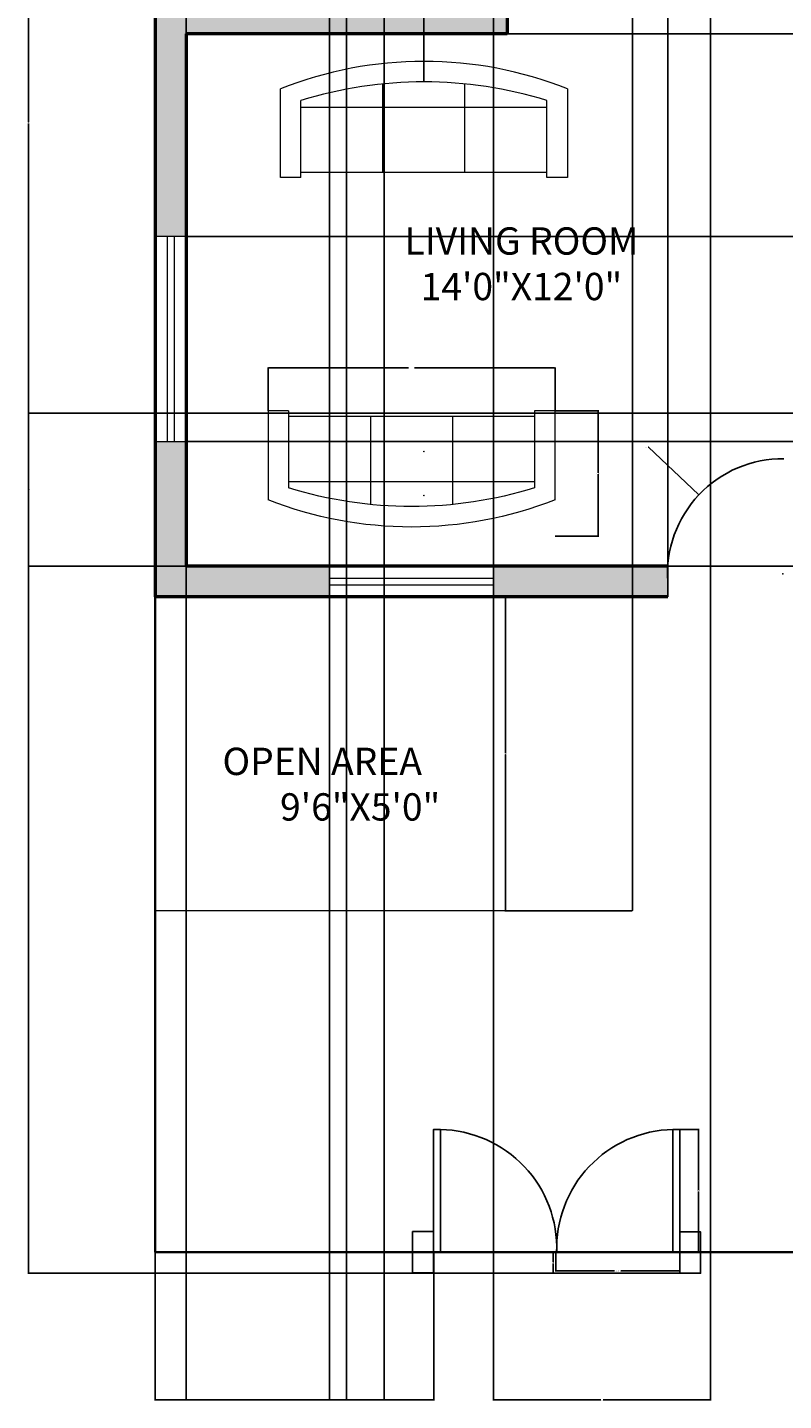
# Model space of a CAD drawing. Units: inches. Extents: x 76 to 532, y 199 to 998.
# Tile 1 of 4: x 123 to 345, y 199 to 601. Entities that reach past the tile are written whole.
import ezdxf

# ---------------------------------------------------------------- set-up
doc = ezdxf.new("R2010")
doc.units = ezdxf.units.IN
for name, color, linetype, lineweight in [('A-ANNO-DIMS', 2, 'Continuous', 18), ('A-AREA-IDEN', 3, 'Continuous', 18), ('A-FURN', 8, 'Continuous', 18), ('A-WALL', 7, 'Continuous', 50), ('A-WALL-PATT', 45, 'Continuous', 13), ('C-PROP', 7, 'Continuous', 35), ('C-SITE', 7, 'Continuous', 18), ('C-SITE-GATE', 1, 'Continuous', 25), ('doors', 1, 'Continuous', 25), ('windows', 140, 'Continuous', 18)]:
    doc.layers.add(name, color=color, linetype=linetype, lineweight=lineweight)
doc.styles.get("Standard").update_dxf_attribs({"font": 'arial.ttf'})
doc.dimstyles.get("Standard").update_dxf_attribs({"dimtxt": 0.18, "dimasz": 0.18, "dimexe": 0.18, "dimexo": 0.0625, "dimgap": 0.09, "dimtad": 0, "dimtih": 1, "dimtoh": 1, "dimdec": 4, "dimzin": 0, "dimdsep": 46, "dimtxsty": 'Standard', "dimcen": 0.09, "dimadec": 0, "dimazin": 0, "dimtfac": 1, "dimtdec": 4, "dimtofl": 0, "dimtmove": 0, "dimatfit": 3, "dimfxl": 1, "dimtolj": 1, "dimtzin": 0, "dimarcsym": 0})

# ---------------------------------------------------------------- blocks, each defined once
blk = doc.blocks.new('Sofa - Roundback 7 ft.')
for p, q in [((-12.00002, -32.4421), (-12.00003, -6.5971)), ((11.99997, -32.4421), (11.99998, -6.5971)), ((-36.000027, -34), (-36.000027, -11.4696)), ((35.99998, -34), (35.99998, -11.4696)), ((-35.999844, -13.3819), (35.9998, -13.3819)), ((-36.000027, -32.4421), (35.99998, -32.4421))]:
    blk.add_line(p, q)
for points in [[(-36.000027, -34), (-42.000027, -34), (-42.000027, -8)], [(41.99998, -8), (41.99998, -34), (35.99998, -34)]]:
    blk.add_lwpolyline(points)
for centre, radius, start, end in [((0, -114.25), 114.25, 68.43141, 111.5686), ((-0.00001, -127.1968), 121.1968, 72.72033, 107.2797)]:
    blk.add_arc(centre, radius, start, end)
blk = doc.blocks.new('WIN-48IN')
for p, q in [((0, 5.5), (48, 5.5)), ((0, 3.5), (48, 3.5))]:
    blk.add_line(p, q)
blk.add_lwpolyline([(0, 0), (48, 0), (48, 9), (0, 9)], close=True)
blk = doc.blocks.new('GATE-LEAF-36IN')
blk.add_lwpolyline([(34, 36), (36, 36), (36, 0), (34, 0)], close=True)
blk.add_arc((34.74, 1.25), 34.76, 91.2122, 182.061)
blk = doc.blocks.new('*D25')
at = {"layer": 'A-ANNO-DIMS', "color": 0, "lineweight": -2, "transparency": 16777216}
for p, q in [((193.86, 488.56), (193.86, 501.28)), ((194.04, 501.1), (234.95, 501.1)), ((277.68, 501.1), (236.76, 501.1)), ((277.86, 488.56), (277.86, 501.28))]:
    blk.add_line(p, q, dxfattribs=at)
at = {"layer": 'A-ANNO-DIMS', "color": 0, "transparency": 16777216}
for points in [[(194.04, 501.13), (194.04, 501.07), (193.86, 501.1)], [(277.68, 501.13), (277.68, 501.07), (277.86, 501.1)]]:
    blk.add_solid(points, dxfattribs=at)
at = {"layer": 'Defpoints', "color": 0, "transparency": 16777216}
for p in [(277.86, 501.1), (193.86, 488.5), (277.86, 488.5)]:
    blk.add_point(p, dxfattribs=at)
at = {"layer": 'A-ANNO-DIMS', "color": 0, "transparency": 16777216, "insert": (235.86, 501.1), "char_height": 0.18, "attachment_point": 5}
blk.add_mtext('\\A1;SOFA 84 TYP.', dxfattribs=at)
blk = doc.blocks.new('*D26')
at = {"layer": 'A-ANNO-DIMS', "color": 0, "lineweight": -2, "transparency": 16777216}
for p, q in [((277.92, 488.5), (290.64, 488.5)), ((290.46, 488.32), (290.46, 470.35)), ((290.46, 452.02), (290.46, 469.99)), ((277.92, 451.84), (290.64, 451.84))]:
    blk.add_line(p, q, dxfattribs=at)
at = {"layer": 'A-ANNO-DIMS', "color": 0, "transparency": 16777216}
for points in [[(290.43, 488.32), (290.49, 488.32), (290.46, 488.5)], [(290.43, 452.02), (290.49, 452.02), (290.46, 451.84)]]:
    blk.add_solid(points, dxfattribs=at)
at = {"layer": 'Defpoints', "color": 0, "transparency": 16777216}
for p in [(277.86, 488.5), (277.86, 451.84), (290.46, 451.84)]:
    blk.add_point(p, dxfattribs=at)
at = {"layer": 'A-ANNO-DIMS', "color": 0, "transparency": 16777216, "insert": (290.46, 470.17), "char_height": 0.18, "attachment_point": 5}
blk.add_mtext('\\A1;37 TYP.', dxfattribs=at)
blk = doc.blocks.new('*D27')
at = {"layer": 'A-ANNO-DIMS', "color": 0, "lineweight": -2, "transparency": 16777216}
for p, q in [((278.05, 241.97), (278.05, 236.4)), ((314.38, 241.97), (314.38, 236.4)), ((278.23, 236.58), (295.31, 236.58)), ((314.2, 236.58), (297.12, 236.58))]:
    blk.add_line(p, q, dxfattribs=at)
at = {"layer": 'A-ANNO-DIMS', "color": 0, "transparency": 16777216}
for points in [[(278.23, 236.61), (278.23, 236.55), (278.05, 236.58)], [(314.2, 236.61), (314.2, 236.55), (314.38, 236.58)]]:
    blk.add_solid(points, dxfattribs=at)
at = {"layer": 'Defpoints', "color": 0, "transparency": 16777216}
for p in [(278.05, 242.03), (314.38, 242.03), (314.38, 236.58)]:
    blk.add_point(p, dxfattribs=at)
at = {"layer": 'A-ANNO-DIMS', "color": 0, "transparency": 16777216, "insert": (296.21, 236.58), "char_height": 0.18, "attachment_point": 5}
blk.add_mtext('\\A1;GATE 36 TYP.', dxfattribs=at)
blk = doc.blocks.new('*D28')
at = {"layer": 'A-ANNO-DIMS', "color": 0, "lineweight": -2, "transparency": 16777216}
for p, q in [((314.44, 278.03), (320.01, 278.03)), ((319.83, 277.85), (319.83, 260.21)), ((319.83, 242.21), (319.83, 259.85)), ((314.44, 242.03), (320.01, 242.03))]:
    blk.add_line(p, q, dxfattribs=at)
at = {"layer": 'A-ANNO-DIMS', "color": 0, "transparency": 16777216}
for points in [[(319.8, 277.85), (319.86, 277.85), (319.83, 278.03)], [(319.8, 242.21), (319.86, 242.21), (319.83, 242.03)]]:
    blk.add_solid(points, dxfattribs=at)
at = {"layer": 'Defpoints', "color": 0, "transparency": 16777216}
for p in [(314.38, 278.03), (319.83, 278.03), (314.38, 242.03)]:
    blk.add_point(p, dxfattribs=at)
at = {"layer": 'A-ANNO-DIMS', "color": 0, "transparency": 16777216, "insert": (319.83, 260.03), "char_height": 0.18, "attachment_point": 5}
blk.add_mtext('\\A1;36 TYP.', dxfattribs=at)
blk = doc.blocks.new('*D32')
at = {"layer": 'A-ANNO-DIMS', "color": 0, "lineweight": -2, "transparency": 16777216}
for p, q in [((160.79, 910.03), (123.58, 910.03)), ((123.76, 909.85), (123.76, 573.14)), ((123.76, 236.06), (123.76, 572.77)), ((320.39, 235.88), (123.58, 235.88))]:
    blk.add_line(p, q, dxfattribs=at)
at = {"layer": 'A-ANNO-DIMS', "color": 0, "transparency": 16777216}
for points in [[(123.73, 909.85), (123.79, 909.85), (123.76, 910.03)], [(123.73, 236.06), (123.79, 236.06), (123.76, 235.88)]]:
    blk.add_solid(points, dxfattribs=at)
at = {"layer": 'Defpoints', "color": 0, "transparency": 16777216}
for p in [(123.76, 910.03), (160.86, 910.03), (320.45, 235.88)]:
    blk.add_point(p, dxfattribs=at)
at = {"layer": 'A-ANNO-DIMS', "color": 0, "transparency": 16777216, "insert": (123.76, 572.95), "char_height": 0.18, "attachment_point": 5}
blk.add_mtext('\\A1;674.1', dxfattribs=at)
blk = doc.blocks.new('*D33')
at = {"layer": 'A-ANNO-DIMS', "color": 0, "lineweight": -2, "transparency": 16777216}
for p, q in [((314.32, 242.03), (277.1, 242.03)), ((277.28, 241.85), (277.28, 239.14)), ((277.28, 236.06), (277.28, 238.77)), ((314.32, 235.88), (277.1, 235.88))]:
    blk.add_line(p, q, dxfattribs=at)
at = {"layer": 'A-ANNO-DIMS', "color": 0, "transparency": 16777216}
for points in [[(277.25, 241.85), (277.31, 241.85), (277.28, 242.03)], [(277.25, 236.06), (277.31, 236.06), (277.28, 235.88)]]:
    blk.add_solid(points, dxfattribs=at)
at = {"layer": 'Defpoints', "color": 0, "transparency": 16777216}
for p in [(277.28, 242.03), (314.38, 242.03), (314.38, 235.88)]:
    blk.add_point(p, dxfattribs=at)
at = {"layer": 'A-ANNO-DIMS', "color": 0, "transparency": 16777216, "insert": (277.28, 238.95), "char_height": 0.18, "attachment_point": 5}
blk.add_mtext('\\A1;6.148', dxfattribs=at)
blk = doc.blocks.new('*D39')
at = {"layer": 'A-ANNO-DIMS', "color": 0, "lineweight": -2, "transparency": 16777216}
for p, q in [((169.86, 900.97), (169.86, 198.6)), ((211.86, 900.97), (211.86, 198.6)), ((170.04, 198.78), (190.64, 198.78)), ((211.68, 198.78), (191.08, 198.78))]:
    blk.add_line(p, q, dxfattribs=at)
at = {"layer": 'A-ANNO-DIMS', "color": 0, "transparency": 16777216}
for points in [[(170.04, 198.81), (170.04, 198.75), (169.86, 198.78)], [(211.68, 198.81), (211.68, 198.75), (211.86, 198.78)]]:
    blk.add_solid(points, dxfattribs=at)
at = {"layer": 'Defpoints', "color": 0, "transparency": 16777216}
for p in [(169.86, 901.03), (211.86, 901.03), (211.86, 198.78)]:
    blk.add_point(p, dxfattribs=at)
at = {"layer": 'A-ANNO-DIMS', "color": 0, "transparency": 16777216, "insert": (190.86, 198.78), "char_height": 0.18, "attachment_point": 5}
blk.add_mtext('\\A1;42', dxfattribs=at)
blk = doc.blocks.new('*D40')
at = {"layer": 'A-ANNO-DIMS', "color": 0, "lineweight": -2, "transparency": 16777216}
for p, q in [((259.86, 900.97), (259.86, 198.6)), ((323.36, 900.97), (323.36, 198.6)), ((260.04, 198.78), (291.28, 198.78)), ((323.18, 198.78), (291.93, 198.78))]:
    blk.add_line(p, q, dxfattribs=at)
at = {"layer": 'A-ANNO-DIMS', "color": 0, "transparency": 16777216}
for points in [[(260.04, 198.81), (260.04, 198.75), (259.86, 198.78)], [(323.18, 198.81), (323.18, 198.75), (323.36, 198.78)]]:
    blk.add_solid(points, dxfattribs=at)
at = {"layer": 'Defpoints', "color": 0, "transparency": 16777216}
for p in [(259.86, 901.03), (323.36, 901.03), (323.36, 198.78)]:
    blk.add_point(p, dxfattribs=at)
at = {"layer": 'A-ANNO-DIMS', "color": 0, "transparency": 16777216, "insert": (291.61, 198.78), "char_height": 0.18, "attachment_point": 5}
blk.add_mtext('\\A1;63.5', dxfattribs=at)
blk = doc.blocks.new('*D42')
at = {"layer": 'A-ANNO-DIMS', "color": 0, "lineweight": -2, "transparency": 16777216}
for p, q in [((160.86, 241.97), (160.86, 198.6)), ((242.34, 241.97), (242.34, 198.6)), ((161.04, 198.78), (201.2, 198.78)), ((242.16, 198.78), (201.99, 198.78))]:
    blk.add_line(p, q, dxfattribs=at)
at = {"layer": 'A-ANNO-DIMS', "color": 0, "transparency": 16777216}
for points in [[(161.04, 198.81), (161.04, 198.75), (160.86, 198.78)], [(242.16, 198.81), (242.16, 198.75), (242.34, 198.78)]]:
    blk.add_solid(points, dxfattribs=at)
at = {"layer": 'Defpoints', "color": 0, "transparency": 16777216}
for p in [(160.86, 242.03), (242.34, 242.03), (242.34, 198.78)]:
    blk.add_point(p, dxfattribs=at)
at = {"layer": 'A-ANNO-DIMS', "color": 0, "transparency": 16777216, "insert": (201.6, 198.78), "char_height": 0.18, "attachment_point": 5}
blk.add_mtext('\\A1;81.48', dxfattribs=at)
blk = doc.blocks.new('*D44')
at = {"layer": 'A-ANNO-DIMS', "color": 0, "lineweight": -2, "transparency": 16777216}
for p, q in [((169.92, 539.57), (532.14, 539.57)), ((531.96, 539.39), (531.96, 509.75)), ((531.96, 479.75), (531.96, 509.39)), ((169.92, 479.57), (532.14, 479.57))]:
    blk.add_line(p, q, dxfattribs=at)
at = {"layer": 'A-ANNO-DIMS', "color": 0, "transparency": 16777216}
for points in [[(531.93, 539.39), (531.99, 539.39), (531.96, 539.57)], [(531.93, 479.75), (531.99, 479.75), (531.96, 479.57)]]:
    blk.add_solid(points, dxfattribs=at)
at = {"layer": 'Defpoints', "color": 0, "transparency": 16777216}
for p in [(169.86, 539.57), (531.96, 539.57), (169.86, 479.57)]:
    blk.add_point(p, dxfattribs=at)
at = {"layer": 'A-ANNO-DIMS', "color": 0, "transparency": 16777216, "insert": (531.96, 509.57), "char_height": 0.18, "attachment_point": 5}
blk.add_mtext('\\A1;60', dxfattribs=at)
blk = doc.blocks.new('*D45')
at = {"layer": 'A-ANNO-DIMS', "color": 0, "lineweight": -2, "transparency": 16777216}
for p, q in [((169.92, 599.03), (532.14, 599.03)), ((531.96, 598.85), (531.96, 569.48)), ((531.96, 539.75), (531.96, 569.12)), ((169.92, 539.57), (532.14, 539.57))]:
    blk.add_line(p, q, dxfattribs=at)
at = {"layer": 'A-ANNO-DIMS', "color": 0, "transparency": 16777216}
for points in [[(531.93, 598.85), (531.99, 598.85), (531.96, 599.03)], [(531.93, 539.75), (531.99, 539.75), (531.96, 539.57)]]:
    blk.add_solid(points, dxfattribs=at)
at = {"layer": 'Defpoints', "color": 0, "transparency": 16777216}
for p in [(169.86, 599.03), (531.96, 599.03), (169.86, 539.57)]:
    blk.add_point(p, dxfattribs=at)
at = {"layer": 'A-ANNO-DIMS', "color": 0, "transparency": 16777216, "insert": (531.96, 569.3), "char_height": 0.18, "attachment_point": 5}
blk.add_mtext('\\A1;59.46', dxfattribs=at)
blk = doc.blocks.new('*D47')
at = {"layer": 'A-ANNO-DIMS', "color": 0, "lineweight": -2, "transparency": 16777216}
for p, q in [((216.86, 727.97), (216.86, 198.6)), ((227.86, 727.97), (227.86, 198.6)), ((217.04, 198.78), (222.16, 198.78)), ((227.68, 198.78), (222.55, 198.78))]:
    blk.add_line(p, q, dxfattribs=at)
at = {"layer": 'A-ANNO-DIMS', "color": 0, "transparency": 16777216}
for points in [[(217.04, 198.81), (217.04, 198.75), (216.86, 198.78)], [(227.68, 198.81), (227.68, 198.75), (227.86, 198.78)]]:
    blk.add_solid(points, dxfattribs=at)
at = {"layer": 'Defpoints', "color": 0, "transparency": 16777216}
for p in [(216.86, 728.03), (227.86, 728.03), (227.86, 198.78)]:
    blk.add_point(p, dxfattribs=at)
at = {"layer": 'A-ANNO-DIMS', "color": 0, "transparency": 16777216, "insert": (222.36, 198.78), "char_height": 0.18, "attachment_point": 5}
blk.add_mtext('\\A1;11', dxfattribs=at)
blk = doc.blocks.new('*D50')
at = {"layer": 'A-ANNO-DIMS', "color": 0, "lineweight": -2, "transparency": 16777216}
for p, q in [((160.86, 433.97), (160.86, 198.6)), ((211.86, 433.97), (211.86, 198.6)), ((161.04, 198.78), (186.16, 198.78)), ((211.68, 198.78), (186.56, 198.78))]:
    blk.add_line(p, q, dxfattribs=at)
at = {"layer": 'A-ANNO-DIMS', "color": 0, "transparency": 16777216}
for points in [[(161.04, 198.81), (161.04, 198.75), (160.86, 198.78)], [(211.68, 198.81), (211.68, 198.75), (211.86, 198.78)]]:
    blk.add_solid(points, dxfattribs=at)
at = {"layer": 'Defpoints', "color": 0, "transparency": 16777216}
for p in [(160.86, 434.03), (211.86, 434.03), (211.86, 198.78)]:
    blk.add_point(p, dxfattribs=at)
at = {"layer": 'A-ANNO-DIMS', "color": 0, "transparency": 16777216, "insert": (186.36, 198.78), "char_height": 0.18, "attachment_point": 5}
blk.add_mtext('\\A1;51', dxfattribs=at)
blk = doc.blocks.new('*D51')
at = {"layer": 'A-ANNO-DIMS', "color": 0, "lineweight": -2, "transparency": 16777216}
for p, q in [((259.86, 443.09), (259.86, 998.31)), ((260.04, 998.13), (285.16, 998.13)), ((310.68, 998.13), (285.56, 998.13)), ((310.86, 443.09), (310.86, 998.31))]:
    blk.add_line(p, q, dxfattribs=at)
at = {"layer": 'A-ANNO-DIMS', "color": 0, "transparency": 16777216}
for points in [[(260.04, 998.16), (260.04, 998.1), (259.86, 998.13)], [(310.68, 998.16), (310.68, 998.1), (310.86, 998.13)]]:
    blk.add_solid(points, dxfattribs=at)
at = {"layer": 'Defpoints', "color": 0, "transparency": 16777216}
for p in [(310.86, 998.13), (259.86, 443.03), (310.86, 443.03)]:
    blk.add_point(p, dxfattribs=at)
at = {"layer": 'A-ANNO-DIMS', "color": 0, "transparency": 16777216, "insert": (285.36, 998.13), "char_height": 0.18, "attachment_point": 5}
blk.add_mtext('\\A1;51', dxfattribs=at)
blk = doc.blocks.new('*D52')
at = {"layer": 'A-ANNO-DIMS', "color": 0, "lineweight": -2, "transparency": 16777216}
for p, q in [((160.86, 342.13), (160.86, 998.31)), ((161.04, 998.13), (230.22, 998.13)), ((300.31, 998.13), (231.13, 998.13)), ((300.49, 342.13), (300.49, 998.31))]:
    blk.add_line(p, q, dxfattribs=at)
at = {"layer": 'A-ANNO-DIMS', "color": 0, "transparency": 16777216}
for points in [[(161.04, 998.16), (161.04, 998.1), (160.86, 998.13)], [(300.31, 998.16), (300.31, 998.1), (300.49, 998.13)]]:
    blk.add_solid(points, dxfattribs=at)
at = {"layer": 'Defpoints', "color": 0, "transparency": 16777216}
for p in [(300.49, 998.13), (160.86, 342.07), (300.49, 342.07)]:
    blk.add_point(p, dxfattribs=at)
at = {"layer": 'A-ANNO-DIMS', "color": 0, "transparency": 16777216, "insert": (230.67, 998.13), "char_height": 0.18, "attachment_point": 5}
blk.add_mtext('\\A1;139.63', dxfattribs=at)
blk = doc.blocks.new('*D53')
at = {"layer": 'A-ANNO-DIMS', "color": 0, "lineweight": -2, "transparency": 16777216}
for p, q in [((300.43, 434.03), (263.21, 434.03)), ((263.39, 433.85), (263.39, 388.23)), ((263.39, 342.25), (263.39, 387.87)), ((300.43, 342.07), (263.21, 342.07))]:
    blk.add_line(p, q, dxfattribs=at)
at = {"layer": 'A-ANNO-DIMS', "color": 0, "transparency": 16777216}
for points in [[(263.36, 433.85), (263.42, 433.85), (263.39, 434.03)], [(263.36, 342.25), (263.42, 342.25), (263.39, 342.07)]]:
    blk.add_solid(points, dxfattribs=at)
at = {"layer": 'Defpoints', "color": 0, "transparency": 16777216}
for p in [(263.39, 434.03), (300.49, 434.03), (300.49, 342.07)]:
    blk.add_point(p, dxfattribs=at)
at = {"layer": 'A-ANNO-DIMS', "color": 0, "transparency": 16777216, "insert": (263.39, 388.05), "char_height": 0.18, "attachment_point": 5}
blk.add_mtext('\\A1;91.96', dxfattribs=at)
blk = doc.blocks.new('*D54')
at = {"layer": 'A-ANNO-DIMS', "color": 0, "lineweight": -2, "transparency": 16777216}
for p, q in [((485.79, 487.86), (123.58, 487.86)), ((123.76, 487.68), (123.76, 465.62)), ((123.76, 443.21), (123.76, 465.26)), ((485.79, 443.03), (123.58, 443.03))]:
    blk.add_line(p, q, dxfattribs=at)
at = {"layer": 'A-ANNO-DIMS', "color": 0, "transparency": 16777216}
for points in [[(123.73, 487.68), (123.79, 487.68), (123.76, 487.86)], [(123.73, 443.21), (123.79, 443.21), (123.76, 443.03)]]:
    blk.add_solid(points, dxfattribs=at)
at = {"layer": 'Defpoints', "color": 0, "transparency": 16777216}
for p in [(123.76, 487.86), (485.86, 487.86), (485.86, 443.03)]:
    blk.add_point(p, dxfattribs=at)
at = {"layer": 'A-ANNO-DIMS', "color": 0, "transparency": 16777216, "insert": (123.76, 465.44), "char_height": 0.18, "attachment_point": 5}
blk.add_mtext('\\A1;44.83', dxfattribs=at)
blk = doc.blocks.new('*D59')
at = {"layer": 'A-ANNO-DIMS', "color": 0, "lineweight": -2, "transparency": 16777216}
for p, q in [((305.09, 477.86), (305.27, 477.86)), ((305.27, 477.86), (319.86, 464.08)), ((344.44, 440.78), (344.62, 440.78)), ((344.53, 440.69), (344.53, 440.87))]:
    blk.add_line(p, q, dxfattribs=at)
at = {"layer": 'A-ANNO-DIMS', "color": 0, "transparency": 16777216}
blk.add_solid([(319.89, 464.1), (319.84, 464.05), (320, 463.95)], dxfattribs=at)
at = {"layer": 'Defpoints', "color": 0, "transparency": 16777216}
for p in [(320, 463.95), (344.53, 440.78)]:
    blk.add_point(p, dxfattribs=at)
at = {"layer": 'A-ANNO-DIMS', "color": 0, "transparency": 16777216, "insert": (304.61, 477.86), "char_height": 0.18, "attachment_point": 5}
blk.add_mtext('\\A1;R33.75', dxfattribs=at)
blk = doc.blocks.new('*D61')
at = {"layer": 'A-ANNO-DIMS', "color": 0, "lineweight": -2, "transparency": 16777216}
for p, q in [((239.33, 657.62), (239.51, 657.62)), ((239.51, 657.62), (239.51, 585.09)), ((239.42, 463.71), (239.6, 463.71)), ((239.51, 463.62), (239.51, 463.8))]:
    blk.add_line(p, q, dxfattribs=at)
at = {"layer": 'A-ANNO-DIMS', "color": 0, "transparency": 16777216}
blk.add_solid([(239.54, 585.09), (239.48, 585.09), (239.51, 584.91)], dxfattribs=at)
at = {"layer": 'Defpoints', "color": 0, "transparency": 16777216}
for p in [(239.51, 584.91), (239.51, 463.71)]:
    blk.add_point(p, dxfattribs=at)
at = {"layer": 'A-ANNO-DIMS', "color": 0, "transparency": 16777216, "insert": (238.85, 657.62), "char_height": 0.18, "attachment_point": 5}
blk.add_mtext('\\A1;R121.2', dxfattribs=at)
blk = doc.blocks.new('*D62')
at = {"layer": 'A-ANNO-DIMS', "color": 0, "lineweight": -2, "transparency": 16777216}
for p, q in [((239.33, 659.46), (239.51, 659.46)), ((239.51, 659.46), (239.51, 591.09)), ((239.42, 476.66), (239.6, 476.66)), ((239.51, 476.57), (239.51, 476.75))]:
    blk.add_line(p, q, dxfattribs=at)
at = {"layer": 'A-ANNO-DIMS', "color": 0, "transparency": 16777216}
blk.add_solid([(239.54, 591.09), (239.48, 591.09), (239.51, 590.91)], dxfattribs=at)
at = {"layer": 'Defpoints', "color": 0, "transparency": 16777216}
for p in [(239.51, 590.91), (239.51, 476.66)]:
    blk.add_point(p, dxfattribs=at)
at = {"layer": 'A-ANNO-DIMS', "color": 0, "transparency": 16777216, "insert": (238.78, 659.46), "char_height": 0.18, "attachment_point": 5}
blk.add_mtext('\\A1;R114.25', dxfattribs=at)

msp = doc.modelspace()

# ---------------------------------------------------------------- hatches: boundary and pattern name
at = {"layer": 'A-WALL-PATT'}
h = msp.add_hatch(color=256, dxfattribs=at)
h.dxf.hatch_style = 1
h.paths.add_polyline_path([(323.3571, 910.0275), (259.8571, 910.0275), (259.8571, 901.0275), (301.8571, 901.0275), (301.8571, 769.0275), (301.8571, 764.0275), (306.8571, 764.0275), (306.8571, 806.0275), (306.8571, 811.0275), (306.8571, 901.0275), (323.3571, 901.0275)])
h.paths.add_polyline_path([(211.8571, 910.0275), (160.8571, 910.0275), (160.8571, 539.5719), (169.8571, 539.5719), (169.8571, 599.0275), (263.8571, 599.0275), (263.8571, 604.0275), (169.8571, 604.0275), (169.8571, 764.0275), (263.8571, 764.0275), (263.8571, 766.5275, -0.0179874), (263.8571, 769.0275), (169.8571, 769.0275), (169.8571, 901.0275), (211.8571, 901.0275)])
h.paths.add_polyline_path([(401.8571, 910.0275), (347.3571, 910.0275), (347.3571, 901.0275), (360.8571, 901.0275), (360.8571, 811.0275), (338.8571, 811.0275, -0.02174236), (338.8571, 808.5275), (338.8571, 806.0275), (360.8571, 806.0275), (360.8571, 764.0275), (365.8571, 764.0275), (365.8571, 836.0275), (397.3621, 836.0275), (397.3621, 841.0275), (365.8571, 841.0275), (365.8571, 901.0275), (401.8571, 901.0275)])
h.paths.add_polyline_path([(169.8571, 479.5719), (160.8571, 479.5719), (160.8571, 434.0275), (211.8571, 434.0275), (211.8571, 443.0275), (169.8571, 443.0275)])
h.paths.add_polyline_path([(310.8571, 443.0275), (259.8571, 443.0275), (259.8571, 434.0275), (310.8571, 434.0275), (310.8571, 438.5275, -0.03336892)])
h.paths.add_polyline_path([(353.8571, 599.0275), (353.8571, 604.0275), (348.8571, 604.0275), (348.8571, 599.0275), (348.8571, 443.0275), (348.8571, 434.0275), (396.8571, 434.0275), (396.8571, 443.0275), (353.8571, 443.0275)])
h.paths.add_polyline_path([(494.8571, 619.5776), (485.8571, 619.5776), (485.8571, 604.0275), (427.8571, 604.0275, -0.02174236), (427.8571, 601.5275), (427.8571, 599.0275), (485.8571, 599.0275), (485.8571, 443.0275), (444.8571, 443.0275), (444.8571, 434.0275), (494.8571, 434.0275)])
h.paths.add_polyline_path([(494.8571, 673.4729), (485.8571, 673.4729), (485.8571, 663.0275), (431.8571, 663.0275), (431.8571, 711.0275), (431.8571, 716.0275), (426.8571, 716.0275), (426.8571, 663.0275), (390.8571, 663.0275), (390.8571, 604.0275), (385.8571, 604.0275), (385.8571, 601.5275, -0.02174236), (385.8571, 599.0275), (395.8571, 599.0275), (395.8571, 604.0275), (395.8571, 658.0275), (430.3571, 658.0275), (430.3571, 659.0275), (451.3571, 659.0275), (451.3571, 658.0275), (485.8571, 658.0275), (485.8571, 643.5776), (494.8571, 643.5776)])
h.paths.add_polyline_path([(494.8571, 752.0275), (485.8571, 752.0275), (485.8571, 716.0275), (463.8571, 716.0275), (463.8571, 713.5275, -0.02174236), (463.8571, 711.0275), (485.8571, 711.0275), (485.8571, 697.4729), (494.8571, 697.4729)])
h.paths.add_polyline_path([(494.8571, 910.0275), (449.8571, 910.0275), (449.8571, 901.0275), (485.8571, 901.0275), (485.8571, 841.0275), (429.3621, 841.0275, -0.02174236), (429.3621, 838.5275), (429.3621, 836.0275), (485.8571, 836.0275), (485.8571, 800.0275), (494.8571, 800.0275)])

# ---------------------------------------------------------------- linework, layer by layer
at = {"layer": 'A-WALL'}
for p, q in [((160.8571, 910.0275), (160.8571, 434.0275)), ((263.8571, 604.0275), (263.8571, 599.0275)), ((169.8571, 599.0275), (169.8571, 443.0275)), ((263.8571, 599.0275), (169.8571, 599.0275)), ((310.8571, 443.0275), (169.8571, 443.0275)), ((310.8571, 434.0275), (160.8571, 434.0275))]:
    msp.add_line(p, q, dxfattribs=at)
at = {"layer": 'C-PROP'}
for p, q in [((160.8571, 242.0275), (160.8571, 434.0275)), ((494.8571, 242.0275), (160.8571, 242.0275))]:
    msp.add_line(p, q, dxfattribs=at)
at = {"layer": 'C-SITE'}
for p, q in [((300.4881, 434.0275), (300.4881, 342.0718)), ((300.4881, 342.0718), (160.8571, 342.0718))]:
    msp.add_line(p, q, dxfattribs=at)
at = {"layer": 'C-SITE-GATE'}
for points in [[(236.1514, 248.0905), (242.3361, 248.0905), (242.3361, 235.9645), (236.1514, 235.9645)], [(314.3811, 248.0051), (320.4491, 248.0051), (320.4491, 235.879), (314.3811, 235.879)]]:
    msp.add_lwpolyline(points, close=True, dxfattribs=at)
at = {"layer": 'doors'}
msp.add_line((310.8571, 443.0275), (310.8571, 434.0275), dxfattribs=at)
msp.add_arc((344.5335, 440.7775), 33.7516, 89.450776, 183.822378, dxfattribs=at)
at = {"layer": 'windows'}
for p, q in [((164.3571, 539.5719), (164.3571, 479.5719)), ((166.3571, 539.5719), (166.3571, 479.5719))]:
    msp.add_line(p, q, dxfattribs=at)
msp.add_lwpolyline([(160.8571, 539.5719), (160.8571, 479.5719), (169.8571, 479.5719), (169.8571, 539.5719)], close=True, dxfattribs=at)

# ---------------------------------------------------------------- block references
at = {"layer": 'A-FURN'}
msp.add_blockref('Sofa - Roundback 7 ft.', (239.5062, 590.9061), dxfattribs=at)
at = {"layer": 'A-FURN', "xscale": -1, "rotation": 180}
msp.add_blockref('Sofa - Roundback 7 ft.', (235.8571, 454.5019), dxfattribs=at)
at = {"layer": 'C-SITE-GATE', "extrusion": (0, 0, -1), "zscale": -1}
msp.add_blockref('GATE-LEAF-36IN', (-278.3361, 242.0275), dxfattribs=at)
at = {"layer": 'C-SITE-GATE'}
msp.add_blockref('GATE-LEAF-36IN', (278.3811, 242.0275), dxfattribs=at)
at = {"layer": 'windows'}
msp.add_blockref('WIN-48IN', (211.8571, 434.0275), dxfattribs=at)

# ---------------------------------------------------------------- texts
at = {"layer": 'A-AREA-IDEN', "char_height": 8, "attachment_point": 1}
for s, insert in [('\\pxqc;LIVING ROOM\\P14\'0"X12\'0"', (227.7257, 542.2989)), ('OPEN AREA\\P\\pxqc;9\'6"X5\'0"', (180.5234, 389.8458))]:
    msp.add_mtext_dynamic_manual_height_columns(s, width=80.600486, gutter_width=12.5, heights=[0], dxfattribs=dict(at, insert=insert))

# ---------------------------------------------------------------- dimensions: what is measured, and where the dimension line sits
at = {"layer": 'A-ANNO-DIMS'}
for base, p1, p2, override, picture, middle in [((300.4881, 998.1275), (160.8571, 342.0718), (300.4881, 342.0718), {"dimdec": 2, "dimlfac": 1, "dimrnd": 0, "dimzin": 0, "dimdsep": 46, "dimlunit": 2}, '*D52', (230.6726, 998.1275)), ((310.8571, 998.1275), (259.8571, 443.0275), (310.8571, 443.0275), {"dimdec": 0, "dimlfac": 1, "dimrnd": 0, "dimzin": 0, "dimdsep": 46, "dimlunit": 2}, '*D51', (285.3571, 998.1275)), ((211.8571, 198.779), (169.8571, 901.0275), (211.8571, 901.0275), {"dimdec": 0, "dimlfac": 1, "dimrnd": 0, "dimzin": 0, "dimdsep": 46, "dimlunit": 2}, '*D39', (190.8571, 198.779)), ((323.3571, 198.779), (259.8571, 901.0275), (323.3571, 901.0275), {"dimdec": 1, "dimlfac": 1, "dimrnd": 0, "dimzin": 0, "dimdsep": 46, "dimlunit": 2}, '*D40', (291.6071, 198.779)), ((227.8571, 198.779), (216.8571, 728.0275), (227.8571, 728.0275), {"dimdec": 0, "dimlfac": 1, "dimrnd": 0, "dimzin": 0, "dimdsep": 46, "dimlunit": 2}, '*D47', (222.3571, 198.779)), ((211.8571, 198.779), (160.8571, 434.0275), (211.8571, 434.0275), {"dimdec": 0, "dimlfac": 1, "dimrnd": 0, "dimzin": 0, "dimdsep": 46, "dimlunit": 2}, '*D50', (186.3571, 198.779)), ((242.3361, 198.779), (160.8571, 242.0275), (242.3361, 242.0275), {"dimdec": 2, "dimlfac": 1, "dimrnd": 0, "dimzin": 0, "dimdsep": 46, "dimlunit": 2}, '*D42', (201.5966, 198.779))]:
    dim = msp.add_linear_dim(base=base, p1=p1, p2=p2, dimstyle='Standard', override=override, dxfattribs=at)
    dim.commit()
    dim.dimension.update_dxf_attribs({"geometry": picture, "text_midpoint": middle})
for base, p1, p2, override, picture, middle in [((123.7571, 910.0275), (320.4491, 235.879), (160.8571, 910.0275), {"dimdec": 1, "dimlfac": 1, "dimrnd": 0, "dimzin": 0, "dimdsep": 46, "dimlunit": 2}, '*D32', (123.7571, 572.9533)), ((531.9571, 599.0275), (169.8571, 539.5719), (169.8571, 599.0275), {"dimdec": 2, "dimlfac": 1, "dimrnd": 0, "dimzin": 0, "dimdsep": 46, "dimlunit": 2}, '*D45', (531.9571, 569.2997)), ((531.9571, 539.5719), (169.8571, 479.5719), (169.8571, 539.5719), {"dimdec": 0, "dimlfac": 1, "dimrnd": 0, "dimzin": 0, "dimdsep": 46, "dimlunit": 2}, '*D44', (531.9571, 509.5719)), ((123.7571, 487.8578), (485.8571, 443.0275), (485.8571, 487.8578), {"dimdec": 2, "dimlfac": 1, "dimrnd": 0, "dimzin": 0, "dimdsep": 46, "dimlunit": 2}, '*D54', (123.7571, 465.4426)), ((263.3881, 434.0275), (300.4881, 342.0718), (300.4881, 434.0275), {"dimdec": 2, "dimlfac": 1, "dimrnd": 0, "dimzin": 0, "dimdsep": 46, "dimlunit": 2}, '*D53', (263.3881, 388.0496)), ((277.28107, 242.02751), (314.38107, 235.87905), (314.38107, 242.02751), {"dimdec": 3, "dimlfac": 1, "dimrnd": 0, "dimzin": 0, "dimdsep": 46, "dimlunit": 2}, '*D33', (277.28107, 238.95328))]:
    dim = msp.add_linear_dim(base=base, p1=p1, p2=p2, angle=90, dimstyle='Standard', override=override, dxfattribs=at)
    dim.commit()
    dim.dimension.update_dxf_attribs({"geometry": picture, "text_midpoint": middle})
for center, mpoint, override, picture, middle in [((239.5062, 476.6561), (239.506, 590.9061), {"dimdec": 2, "dimlfac": 1, "dimrnd": 0, "dimzin": 0, "dimdsep": 46, "dimlunit": 2}, '*D62', (238.7755, 659.4561)), ((239.5062, 463.7093), (239.506, 584.9061), {"dimdec": 1, "dimlfac": 1, "dimrnd": 0, "dimzin": 0, "dimdsep": 46, "dimlunit": 2}, '*D61', (238.847, 657.6242)), ((344.5335, 440.7775), (319.9958, 463.9522), {"dimdec": 2, "dimlfac": 1, "dimrnd": 0, "dimzin": 0, "dimdsep": 46, "dimlunit": 2}, '*D59', (304.6126, 477.857))]:
    dim = msp.add_radius_dim(center=center, mpoint=mpoint, dimstyle='Standard', override=override, dxfattribs=at)
    dim.commit()
    dim.dimension.update_dxf_attribs({"geometry": picture, "text_midpoint": middle, "dimtype": 164})
for base, p1, p2, text, picture, middle in [((277.857, 501.1019), (193.857, 488.5019), (277.857, 488.5019), 'SOFA <> TYP.', '*D25', (235.857, 501.1019)), ((314.3811, 236.5773), (278.0463, 242.0275), (314.3811, 242.0275), 'GATE <> TYP.', '*D27', (296.2137, 236.5773))]:
    dim = msp.add_linear_dim(base=base, p1=p1, p2=p2, text=text, dimstyle='Standard', override={"dimdec": 0, "dimlfac": 1, "dimrnd": 0, "dimzin": 0, "dimdsep": 46, "dimlunit": 2}, dxfattribs=at)
    dim.commit()
    dim.dimension.update_dxf_attribs({"geometry": picture, "text_midpoint": middle})
for base, p1, p2, angle, picture, middle in [((290.457, 451.8353), (277.857, 488.5019), (277.857, 451.8353), 270, '*D26', (290.457, 470.1686)), ((319.8313, 278.0275), (314.3811, 242.0275), (314.3811, 278.0275), 90, '*D28', (319.8313, 260.0275))]:
    dim = msp.add_linear_dim(base=base, p1=p1, p2=p2, angle=angle, text='<> TYP.', dimstyle='Standard', override={"dimdec": 0, "dimlfac": 1, "dimrnd": 0, "dimzin": 0, "dimdsep": 46, "dimlunit": 2}, dxfattribs=at)
    dim.commit()
    dim.dimension.update_dxf_attribs({"geometry": picture, "text_midpoint": middle})

doc.saveas('drawing.dxf')
